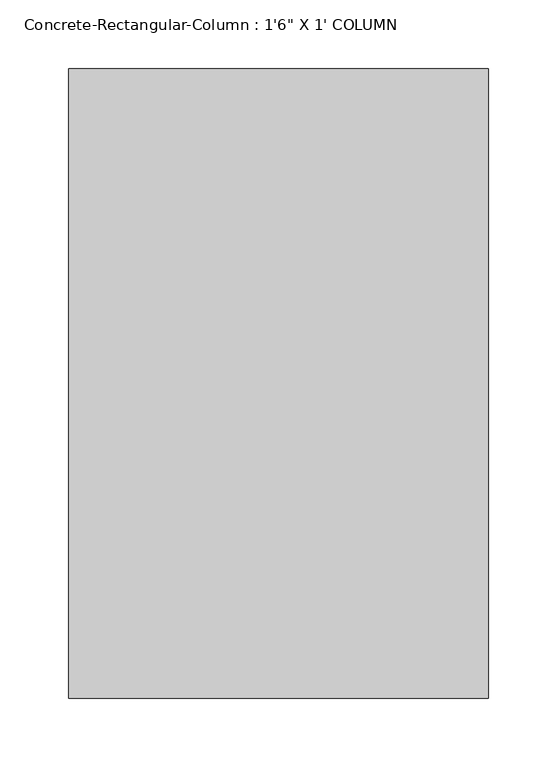
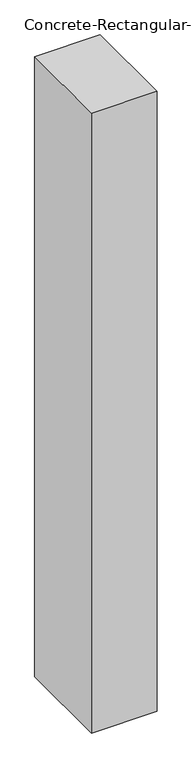
"""IFC4 building model written with IfcOpenShell, lengths in millimetres: column geometry."""

from ifc_helpers import new_model, si_unit, frame, origin, place, context, project, spatial, polyline, outline, extrude, source, transform, mapped, element, save


def column_61ecc76d(model_context):
    return source(origin(), model_context, "Body", "SweptSolid", [
        extrude(outline(polyline([(152.4, 228.6), (152.4, -228.6), (-152.4, -228.6), (-152.4, 228.6), (152.4, 228.6)])), frame((0.0, 0.0, 6400.8), z_axis=(0.0, 0.0, 1.0), x_axis=(1.0, 0.0, 0.0)), (0.0, 0.0, 1.0), 3048.0),
    ])


if __name__ == "__main__":
    model = new_model("IFC4")
    model_context = context("Model", 3, world=origin())
    ifc_project = project(units=[si_unit("LENGTHUNIT", "METRE", prefix="MILLI")], contexts=[model_context])
    site = spatial("IfcSite", under=ifc_project)
    building = spatial("IfcBuilding", under=site)
    placement = place(None, origin())
    column_shape = column_61ecc76d(model_context)
    element("IfcColumn", 1, ObjectType="Concrete-Rectangular-Column : 1'6\" X 1' COLUMN", at=placement, inside=building, context=model_context, shape_type="MappedRepresentation", body=[
        mapped(column_shape, transform((0.0, 0.0, 0.0), x_axis=(1.0, 0.0, 0.0), y_axis=(0.0, 1.0, 0.0), z_axis=(0.0, 0.0, 1.0))),
    ])
    save(model, "model.ifc")

# Revit data of these elements
# Type "Concrete-Rectangular-Column : 1'6\" X 1' COLUMN"
#   Assembly Code = "B10"
#   b = 1' - 0"
#   h = 1' - 6"
#   Structural Material [instance default] = Concrete, Cast-in-Place gray
# Element 1 (IfcColumn, "Concrete-Rectangular-Column : 1'6\" X 1' COLUMN")
#   Structural Material = WARM BEIGE COLOUR
#   Materials on its faces: "WARM BEIGE COLOUR"
# Materials
#   "Concrete, Cast-in-Place gray": class "Concrete", colour RGB 192 192 192, transparency 0, Description = "Cast-in-place concrete", Cost = 0
#   "WARM BEIGE COLOUR": class "Generic", colour RGB 120 120 120, transparency 0, Cost = 0
